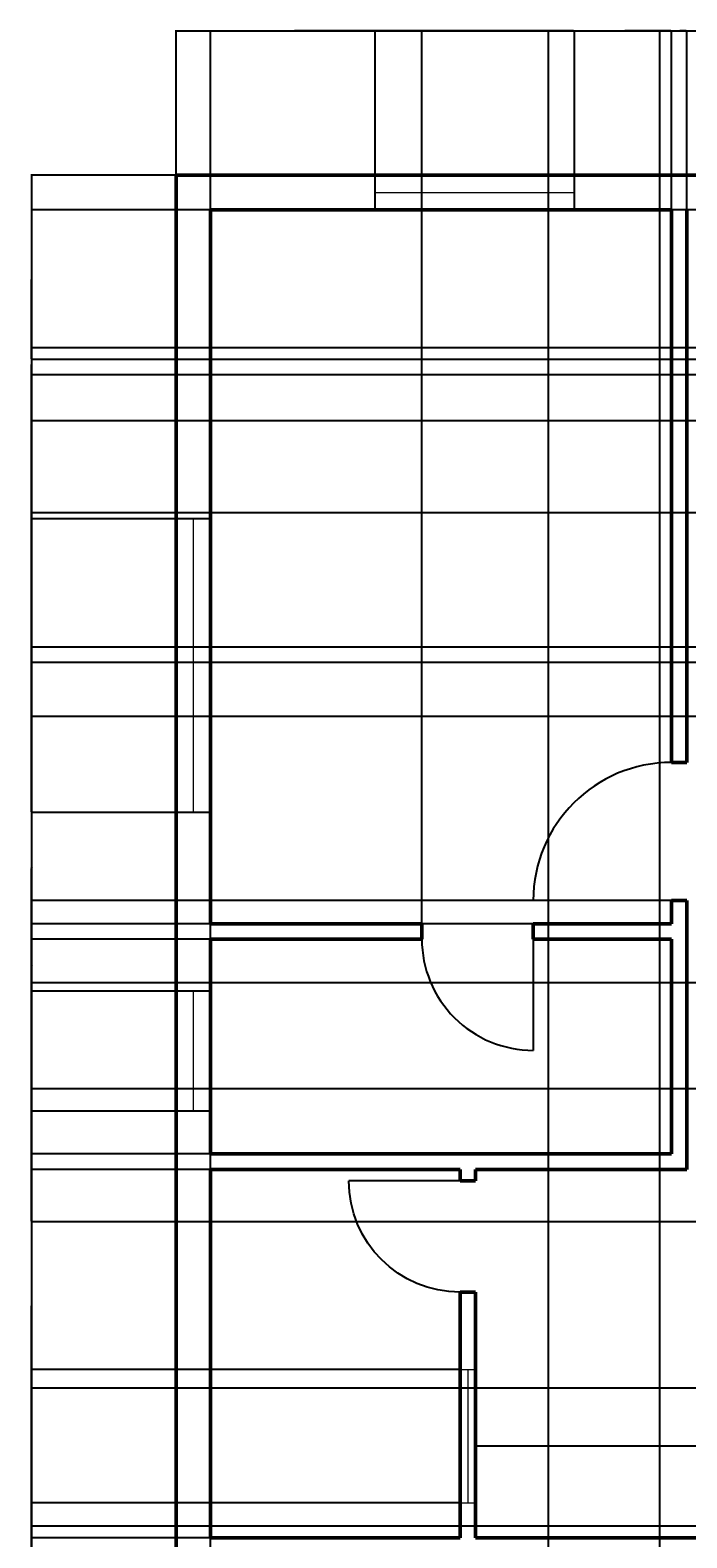
# Model space of a CAD drawing. Units: inches. Extents: x 2479 to 3284, y 2154 to 2936.
# Tile 3 of 8: x 2479 to 2650, y 2543 to 2936. Entities that reach past the tile are written whole.
import ezdxf

# ---------------------------------------------------------------- set-up
doc = ezdxf.new("R2010")
doc.units = ezdxf.units.IN
for name, color, linetype, lineweight in [('A-ANNO-DIMS', 2, 'Continuous', 18), ('A-DOOR', 3, 'Continuous', 25), ('A-FLOR-CASE', 8, 'Continuous', 18), ('A-GLAZ', 4, 'Continuous', 18), ('A-WALL', 7, 'Continuous', 50)]:
    doc.layers.add(name, color=color, linetype=linetype, lineweight=lineweight)
doc.styles.get("Standard").update_dxf_attribs({"font": 'arial.ttf'})
doc.dimstyles.get("Standard").update_dxf_attribs({"dimtxt": 0.18, "dimasz": 0.18, "dimexe": 0.18, "dimexo": 0.0625, "dimgap": 0.09, "dimtad": 0, "dimtih": 1, "dimtoh": 1, "dimdec": 4, "dimzin": 0, "dimdsep": 46, "dimtxsty": 'Standard', "dimcen": 0.09, "dimadec": 0, "dimazin": 0, "dimtfac": 1, "dimtdec": 4, "dimtofl": 0, "dimtmove": 0, "dimatfit": 3, "dimfxl": 1, "dimtolj": 1, "dimtzin": 0, "dimarcsym": 0})

# ---------------------------------------------------------------- blocks, each defined once
blk = doc.blocks.new('DOOR-SWING-29IN')
blk.add_line((29, 0), (0, 0))
blk.add_arc((29, 0), 29, 90, 180)
blk = doc.blocks.new('DOOR-SWING-36IN')
blk.add_line((36, 0), (0, 0))
blk.add_arc((36, 0), 36, 90, 180)
blk = doc.blocks.new('*D8')
at = {"layer": 'A-ANNO-DIMS', "color": 0, "lineweight": -2, "transparency": 16777216}
for p, q in [((2517.15, 2897.74), (2479.43, 2897.74)), ((2479.61, 2897.56), (2479.61, 2544.92)), ((2479.61, 2191.92), (2479.61, 2544.56)), ((2517.15, 2191.74), (2479.43, 2191.74))]:
    blk.add_line(p, q, dxfattribs=at)
at = {"layer": 'A-ANNO-DIMS', "color": 0, "transparency": 16777216}
for points in [[(2479.58, 2897.56), (2479.64, 2897.56), (2479.61, 2897.74)], [(2479.58, 2191.92), (2479.64, 2191.92), (2479.61, 2191.74)]]:
    blk.add_solid(points, dxfattribs=at)
at = {"layer": 'Defpoints', "color": 0, "transparency": 16777216}
for p in [(2479.61, 2897.74), (2517.21, 2897.74), (2517.21, 2191.74)]:
    blk.add_point(p, dxfattribs=at)
at = {"layer": 'A-ANNO-DIMS', "color": 0, "transparency": 16777216, "insert": (2479.61, 2544.74), "char_height": 0.18, "attachment_point": 5}
blk.add_mtext('\\A1;706', dxfattribs=at)
blk = doc.blocks.new('*D9')
at = {"layer": 'A-ANNO-DIMS', "color": 0, "lineweight": -2, "transparency": 16777216}
for p, q in [((2517.21, 2897.8), (2517.21, 2935.52)), ((2517.39, 2935.34), (2710.92, 2935.34)), ((2905.03, 2935.34), (2711.5, 2935.34)), ((2905.21, 2888.8), (2905.21, 2935.52))]:
    blk.add_line(p, q, dxfattribs=at)
at = {"layer": 'A-ANNO-DIMS', "color": 0, "transparency": 16777216}
for points in [[(2517.39, 2935.37), (2517.39, 2935.31), (2517.21, 2935.34)], [(2905.03, 2935.37), (2905.03, 2935.31), (2905.21, 2935.34)]]:
    blk.add_solid(points, dxfattribs=at)
at = {"layer": 'Defpoints', "color": 0, "transparency": 16777216}
for p in [(2905.21, 2935.34), (2517.21, 2897.74), (2905.21, 2888.74)]:
    blk.add_point(p, dxfattribs=at)
at = {"layer": 'A-ANNO-DIMS', "color": 0, "transparency": 16777216, "insert": (2711.21, 2935.34), "char_height": 0.18, "attachment_point": 5}
blk.add_mtext('\\A1;388', dxfattribs=at)
blk = doc.blocks.new('*D27')
at = {"layer": 'A-ANNO-DIMS', "color": 0, "lineweight": -2, "transparency": 16777216}
for p, q in [((2845.15, 2545.74), (2479.43, 2545.74)), ((2479.61, 2545.56), (2479.61, 2536.92)), ((2479.61, 2527.92), (2479.61, 2536.56)), ((2845.15, 2527.74), (2479.43, 2527.74))]:
    blk.add_line(p, q, dxfattribs=at)
at = {"layer": 'A-ANNO-DIMS', "color": 0, "transparency": 16777216}
for points in [[(2479.58, 2545.56), (2479.64, 2545.56), (2479.61, 2545.74)], [(2479.58, 2527.92), (2479.64, 2527.92), (2479.61, 2527.74)]]:
    blk.add_solid(points, dxfattribs=at)
at = {"layer": 'Defpoints', "color": 0, "transparency": 16777216}
for p in [(2479.61, 2545.74), (2845.21, 2545.74), (2845.21, 2527.74)]:
    blk.add_point(p, dxfattribs=at)
at = {"layer": 'A-ANNO-DIMS', "color": 0, "transparency": 16777216, "insert": (2479.61, 2536.74), "char_height": 0.18, "attachment_point": 5}
blk.add_mtext('\\A1;18', dxfattribs=at)
blk = doc.blocks.new('*D28')
at = {"layer": 'A-ANNO-DIMS', "color": 0, "lineweight": -2, "transparency": 16777216}
for p, q in [((2845.15, 2625.04), (2479.43, 2625.04)), ((2479.61, 2624.86), (2479.61, 2603.57)), ((2479.61, 2581.92), (2479.61, 2603.21)), ((2845.15, 2581.74), (2479.43, 2581.74))]:
    blk.add_line(p, q, dxfattribs=at)
at = {"layer": 'A-ANNO-DIMS', "color": 0, "transparency": 16777216}
for points in [[(2479.58, 2624.86), (2479.64, 2624.86), (2479.61, 2625.04)], [(2479.58, 2581.92), (2479.64, 2581.92), (2479.61, 2581.74)]]:
    blk.add_solid(points, dxfattribs=at)
at = {"layer": 'Defpoints', "color": 0, "transparency": 16777216}
for p in [(2479.61, 2625.04), (2845.21, 2625.04), (2845.21, 2581.74)]:
    blk.add_point(p, dxfattribs=at)
at = {"layer": 'A-ANNO-DIMS', "color": 0, "transparency": 16777216, "insert": (2479.61, 2603.39), "char_height": 0.18, "attachment_point": 5}
blk.add_mtext('\\A1;43.3', dxfattribs=at)
blk = doc.blocks.new('*D29')
at = {"layer": 'A-ANNO-DIMS', "color": 0, "lineweight": -2, "transparency": 16777216}
for p, q in [((2845.15, 2687.36), (2479.43, 2687.36)), ((2479.61, 2687.18), (2479.61, 2656.38)), ((2479.61, 2625.22), (2479.61, 2656.01)), ((2845.15, 2625.04), (2479.43, 2625.04))]:
    blk.add_line(p, q, dxfattribs=at)
at = {"layer": 'A-ANNO-DIMS', "color": 0, "transparency": 16777216}
for points in [[(2479.58, 2687.18), (2479.64, 2687.18), (2479.61, 2687.36)], [(2479.58, 2625.22), (2479.64, 2625.22), (2479.61, 2625.04)]]:
    blk.add_solid(points, dxfattribs=at)
at = {"layer": 'Defpoints', "color": 0, "transparency": 16777216}
for p in [(2479.61, 2687.36), (2845.21, 2687.36), (2845.21, 2625.04)]:
    blk.add_point(p, dxfattribs=at)
at = {"layer": 'A-ANNO-DIMS', "color": 0, "transparency": 16777216, "insert": (2479.61, 2656.2), "char_height": 0.18, "attachment_point": 5}
blk.add_mtext('\\A1;62.32', dxfattribs=at)
blk = doc.blocks.new('*D30')
at = {"layer": 'A-ANNO-DIMS', "color": 0, "lineweight": -2, "transparency": 16777216}
for p, q in [((2845.15, 2852.74), (2479.43, 2852.74)), ((2479.61, 2852.56), (2479.61, 2804.92)), ((2479.61, 2756.92), (2479.61, 2804.56)), ((2845.15, 2756.74), (2479.43, 2756.74))]:
    blk.add_line(p, q, dxfattribs=at)
at = {"layer": 'A-ANNO-DIMS', "color": 0, "transparency": 16777216}
for points in [[(2479.58, 2852.56), (2479.64, 2852.56), (2479.61, 2852.74)], [(2479.58, 2756.92), (2479.64, 2756.92), (2479.61, 2756.74)]]:
    blk.add_solid(points, dxfattribs=at)
at = {"layer": 'Defpoints', "color": 0, "transparency": 16777216}
for p in [(2479.61, 2852.74), (2845.21, 2852.74), (2845.21, 2756.74)]:
    blk.add_point(p, dxfattribs=at)
at = {"layer": 'A-ANNO-DIMS', "color": 0, "transparency": 16777216, "insert": (2479.61, 2804.74), "char_height": 0.18, "attachment_point": 5}
blk.add_mtext('\\A1;96', dxfattribs=at)
blk = doc.blocks.new('*D31')
at = {"layer": 'A-ANNO-DIMS', "color": 0, "lineweight": -2, "transparency": 16777216}
for p, q in [((2845.15, 2888.74), (2479.43, 2888.74)), ((2479.61, 2888.56), (2479.61, 2870.92)), ((2479.61, 2852.92), (2479.61, 2870.56)), ((2845.15, 2852.74), (2479.43, 2852.74))]:
    blk.add_line(p, q, dxfattribs=at)
at = {"layer": 'A-ANNO-DIMS', "color": 0, "transparency": 16777216}
for points in [[(2479.58, 2888.56), (2479.64, 2888.56), (2479.61, 2888.74)], [(2479.58, 2852.92), (2479.64, 2852.92), (2479.61, 2852.74)]]:
    blk.add_solid(points, dxfattribs=at)
at = {"layer": 'Defpoints', "color": 0, "transparency": 16777216}
for p in [(2479.61, 2888.74), (2845.21, 2888.74), (2845.21, 2852.74)]:
    blk.add_point(p, dxfattribs=at)
at = {"layer": 'A-ANNO-DIMS', "color": 0, "transparency": 16777216, "insert": (2479.61, 2870.74), "char_height": 0.18, "attachment_point": 5}
blk.add_mtext('\\A1;36', dxfattribs=at)
blk = doc.blocks.new('*D37')
at = {"layer": 'A-ANNO-DIMS', "color": 0, "lineweight": -2, "transparency": 16777216}
for p, q in [((2526.21, 2888.8), (2526.21, 2935.52)), ((2526.39, 2935.34), (2547.16, 2935.34)), ((2568.86, 2935.34), (2548.09, 2935.34)), ((2569.04, 2888.8), (2569.04, 2935.52))]:
    blk.add_line(p, q, dxfattribs=at)
at = {"layer": 'A-ANNO-DIMS', "color": 0, "transparency": 16777216}
for points in [[(2526.39, 2935.37), (2526.39, 2935.31), (2526.21, 2935.34)], [(2568.86, 2935.37), (2568.86, 2935.31), (2569.04, 2935.34)]]:
    blk.add_solid(points, dxfattribs=at)
at = {"layer": 'Defpoints', "color": 0, "transparency": 16777216}
for p in [(2569.04, 2935.34), (2526.21, 2888.74), (2569.04, 2888.74)]:
    blk.add_point(p, dxfattribs=at)
at = {"layer": 'A-ANNO-DIMS', "color": 0, "transparency": 16777216, "insert": (2547.63, 2935.34), "char_height": 0.18, "attachment_point": 5}
blk.add_mtext('\\A1;42.835', dxfattribs=at)
blk = doc.blocks.new('*D38')
at = {"layer": 'A-ANNO-DIMS', "color": 0, "lineweight": -2, "transparency": 16777216}
for p, q in [((2569.04, 2888.8), (2569.04, 2935.52)), ((2569.22, 2935.34), (2594.59, 2935.34)), ((2620.74, 2935.34), (2595.38, 2935.34)), ((2620.92, 2888.8), (2620.92, 2935.52))]:
    blk.add_line(p, q, dxfattribs=at)
at = {"layer": 'A-ANNO-DIMS', "color": 0, "transparency": 16777216}
for points in [[(2569.22, 2935.37), (2569.22, 2935.31), (2569.04, 2935.34)], [(2620.74, 2935.37), (2620.74, 2935.31), (2620.92, 2935.34)]]:
    blk.add_solid(points, dxfattribs=at)
at = {"layer": 'Defpoints', "color": 0, "transparency": 16777216}
for p in [(2620.92, 2935.34), (2569.04, 2888.74), (2620.92, 2888.74)]:
    blk.add_point(p, dxfattribs=at)
at = {"layer": 'A-ANNO-DIMS', "color": 0, "transparency": 16777216, "insert": (2594.98, 2935.34), "char_height": 0.18, "attachment_point": 5}
blk.add_mtext('\\A1;51.88', dxfattribs=at)
blk = doc.blocks.new('*D39')
at = {"layer": 'A-ANNO-DIMS', "color": 0, "lineweight": -2, "transparency": 16777216}
for p, q in [((2620.92, 2888.8), (2620.92, 2935.52)), ((2621.1, 2935.34), (2633.1, 2935.34)), ((2646.03, 2935.34), (2634.03, 2935.34)), ((2646.21, 2888.8), (2646.21, 2935.52))]:
    blk.add_line(p, q, dxfattribs=at)
at = {"layer": 'A-ANNO-DIMS', "color": 0, "transparency": 16777216}
for points in [[(2621.1, 2935.37), (2621.1, 2935.31), (2620.92, 2935.34)], [(2646.03, 2935.37), (2646.03, 2935.31), (2646.21, 2935.34)]]:
    blk.add_solid(points, dxfattribs=at)
at = {"layer": 'Defpoints', "color": 0, "transparency": 16777216}
for p in [(2646.21, 2935.34), (2620.92, 2888.74), (2646.21, 2888.74)]:
    blk.add_point(p, dxfattribs=at)
at = {"layer": 'A-ANNO-DIMS', "color": 0, "transparency": 16777216, "insert": (2633.57, 2935.34), "char_height": 0.18, "attachment_point": 5}
blk.add_mtext('\\A1;25.285', dxfattribs=at)
blk = doc.blocks.new('*D40')
at = {"layer": 'A-ANNO-DIMS', "color": 0, "lineweight": -2, "transparency": 16777216}
for p, q in [((2646.21, 2888.8), (2646.21, 2935.52)), ((2646.39, 2935.34), (2648.06, 2935.34)), ((2650.03, 2935.34), (2648.36, 2935.34)), ((2650.21, 2888.8), (2650.21, 2935.52))]:
    blk.add_line(p, q, dxfattribs=at)
at = {"layer": 'A-ANNO-DIMS', "color": 0, "transparency": 16777216}
for points in [[(2646.39, 2935.37), (2646.39, 2935.31), (2646.21, 2935.34)], [(2650.03, 2935.37), (2650.03, 2935.31), (2650.21, 2935.34)]]:
    blk.add_solid(points, dxfattribs=at)
at = {"layer": 'Defpoints', "color": 0, "transparency": 16777216}
for p in [(2650.21, 2935.34), (2646.21, 2888.74), (2650.21, 2888.74)]:
    blk.add_point(p, dxfattribs=at)
at = {"layer": 'A-ANNO-DIMS', "color": 0, "transparency": 16777216, "insert": (2648.21, 2935.34), "char_height": 0.18, "attachment_point": 5}
blk.add_mtext('\\A1;4', dxfattribs=at)
blk = doc.blocks.new('*D51')
at = {"layer": 'A-ANNO-DIMS', "color": 0, "lineweight": -2, "transparency": 16777216}
for p, q in [((2526.15, 2638.74), (2479.43, 2638.74)), ((2479.61, 2638.56), (2479.61, 2590.92)), ((2479.61, 2542.92), (2479.61, 2590.56)), ((2526.15, 2542.74), (2479.43, 2542.74))]:
    blk.add_line(p, q, dxfattribs=at)
at = {"layer": 'A-ANNO-DIMS', "color": 0, "transparency": 16777216}
for points in [[(2479.58, 2638.56), (2479.64, 2638.56), (2479.61, 2638.74)], [(2479.58, 2542.92), (2479.64, 2542.92), (2479.61, 2542.74)]]:
    blk.add_solid(points, dxfattribs=at)
at = {"layer": 'Defpoints', "color": 0, "transparency": 16777216}
for p in [(2479.61, 2638.74), (2526.21, 2638.74), (2526.21, 2542.74)]:
    blk.add_point(p, dxfattribs=at)
at = {"layer": 'A-ANNO-DIMS', "color": 0, "transparency": 16777216, "insert": (2479.61, 2590.74), "char_height": 0.18, "attachment_point": 5}
blk.add_mtext('\\A1;96', dxfattribs=at)
blk = doc.blocks.new('*D52')
at = {"layer": 'A-ANNO-DIMS', "color": 0, "lineweight": -2, "transparency": 16777216}
for p, q in [((2526.15, 2653.92), (2479.43, 2653.92)), ((2479.61, 2653.74), (2479.61, 2648.51)), ((2479.61, 2642.92), (2479.61, 2648.15)), ((2526.15, 2642.74), (2479.43, 2642.74))]:
    blk.add_line(p, q, dxfattribs=at)
at = {"layer": 'A-ANNO-DIMS', "color": 0, "transparency": 16777216}
for points in [[(2479.58, 2653.74), (2479.64, 2653.74), (2479.61, 2653.92)], [(2479.58, 2642.92), (2479.64, 2642.92), (2479.61, 2642.74)]]:
    blk.add_solid(points, dxfattribs=at)
at = {"layer": 'Defpoints', "color": 0, "transparency": 16777216}
for p in [(2479.61, 2653.92), (2526.21, 2653.92), (2526.21, 2642.74)]:
    blk.add_point(p, dxfattribs=at)
at = {"layer": 'A-ANNO-DIMS', "color": 0, "transparency": 16777216, "insert": (2479.61, 2648.33), "char_height": 0.18, "attachment_point": 5}
blk.add_mtext('\\A1;11.18', dxfattribs=at)
blk = doc.blocks.new('*D53')
at = {"layer": 'A-ANNO-DIMS', "color": 0, "lineweight": -2, "transparency": 16777216}
for p, q in [((2526.15, 2685.18), (2479.43, 2685.18)), ((2479.61, 2685), (2479.61, 2669.73)), ((2479.61, 2654.1), (2479.61, 2669.37)), ((2526.15, 2653.92), (2479.43, 2653.92))]:
    blk.add_line(p, q, dxfattribs=at)
at = {"layer": 'A-ANNO-DIMS', "color": 0, "transparency": 16777216}
for points in [[(2479.58, 2685), (2479.64, 2685), (2479.61, 2685.18)], [(2479.58, 2654.1), (2479.64, 2654.1), (2479.61, 2653.92)]]:
    blk.add_solid(points, dxfattribs=at)
at = {"layer": 'Defpoints', "color": 0, "transparency": 16777216}
for p in [(2479.61, 2685.18), (2526.21, 2685.18), (2526.21, 2653.92)]:
    blk.add_point(p, dxfattribs=at)
at = {"layer": 'A-ANNO-DIMS', "color": 0, "transparency": 16777216, "insert": (2479.61, 2669.55), "char_height": 0.18, "attachment_point": 5}
blk.add_mtext('\\A1;31.26', dxfattribs=at)
blk = doc.blocks.new('*D54')
at = {"layer": 'A-ANNO-DIMS', "color": 0, "lineweight": -2, "transparency": 16777216}
for p, q in [((2526.15, 2698.74), (2479.43, 2698.74)), ((2479.61, 2698.56), (2479.61, 2692.14)), ((2479.61, 2685.36), (2479.61, 2691.78)), ((2526.15, 2685.18), (2479.43, 2685.18))]:
    blk.add_line(p, q, dxfattribs=at)
at = {"layer": 'A-ANNO-DIMS', "color": 0, "transparency": 16777216}
for points in [[(2479.58, 2698.56), (2479.64, 2698.56), (2479.61, 2698.74)], [(2479.58, 2685.36), (2479.64, 2685.36), (2479.61, 2685.18)]]:
    blk.add_solid(points, dxfattribs=at)
at = {"layer": 'Defpoints', "color": 0, "transparency": 16777216}
for p in [(2479.61, 2698.74), (2526.21, 2698.74), (2526.21, 2685.18)]:
    blk.add_point(p, dxfattribs=at)
at = {"layer": 'A-ANNO-DIMS', "color": 0, "transparency": 16777216, "insert": (2479.61, 2691.96), "char_height": 0.18, "attachment_point": 5}
blk.add_mtext('\\A1;13.557', dxfattribs=at)
blk = doc.blocks.new('*D55')
at = {"layer": 'A-ANNO-DIMS', "color": 0, "lineweight": -2, "transparency": 16777216}
for p, q in [((2526.15, 2731.68), (2479.43, 2731.68)), ((2479.61, 2731.5), (2479.61, 2717.39)), ((2479.61, 2702.92), (2479.61, 2717.03)), ((2526.15, 2702.74), (2479.43, 2702.74))]:
    blk.add_line(p, q, dxfattribs=at)
at = {"layer": 'A-ANNO-DIMS', "color": 0, "transparency": 16777216}
for points in [[(2479.58, 2731.5), (2479.64, 2731.5), (2479.61, 2731.68)], [(2479.58, 2702.92), (2479.64, 2702.92), (2479.61, 2702.74)]]:
    blk.add_solid(points, dxfattribs=at)
at = {"layer": 'Defpoints', "color": 0, "transparency": 16777216}
for p in [(2479.61, 2731.68), (2526.21, 2731.68), (2526.21, 2702.74)]:
    blk.add_point(p, dxfattribs=at)
at = {"layer": 'A-ANNO-DIMS', "color": 0, "transparency": 16777216, "insert": (2479.61, 2717.21), "char_height": 0.18, "attachment_point": 5}
blk.add_mtext('\\A1;28.935', dxfattribs=at)
blk = doc.blocks.new('*D56')
at = {"layer": 'A-ANNO-DIMS', "color": 0, "lineweight": -2, "transparency": 16777216}
for p, q in [((2526.15, 2808.2), (2479.43, 2808.2)), ((2479.61, 2808.02), (2479.61, 2770.12)), ((2479.61, 2731.86), (2479.61, 2769.75)), ((2526.15, 2731.68), (2479.43, 2731.68))]:
    blk.add_line(p, q, dxfattribs=at)
at = {"layer": 'A-ANNO-DIMS', "color": 0, "transparency": 16777216}
for points in [[(2479.58, 2808.02), (2479.64, 2808.02), (2479.61, 2808.2)], [(2479.58, 2731.86), (2479.64, 2731.86), (2479.61, 2731.68)]]:
    blk.add_solid(points, dxfattribs=at)
at = {"layer": 'Defpoints', "color": 0, "transparency": 16777216}
for p in [(2479.61, 2808.2), (2526.21, 2808.2), (2526.21, 2731.68)]:
    blk.add_point(p, dxfattribs=at)
at = {"layer": 'A-ANNO-DIMS', "color": 0, "transparency": 16777216, "insert": (2479.61, 2769.94), "char_height": 0.18, "attachment_point": 5}
blk.add_mtext('\\A1;76.52', dxfattribs=at)
blk = doc.blocks.new('*D57')
at = {"layer": 'A-ANNO-DIMS', "color": 0, "lineweight": -2, "transparency": 16777216}
for p, q in [((2526.15, 2888.74), (2479.43, 2888.74)), ((2479.61, 2888.56), (2479.61, 2848.65)), ((2479.61, 2808.38), (2479.61, 2848.29)), ((2526.15, 2808.2), (2479.43, 2808.2))]:
    blk.add_line(p, q, dxfattribs=at)
at = {"layer": 'A-ANNO-DIMS', "color": 0, "transparency": 16777216}
for points in [[(2479.58, 2888.56), (2479.64, 2888.56), (2479.61, 2888.74)], [(2479.58, 2808.38), (2479.64, 2808.38), (2479.61, 2808.2)]]:
    blk.add_solid(points, dxfattribs=at)
at = {"layer": 'Defpoints', "color": 0, "transparency": 16777216}
for p in [(2479.61, 2888.74), (2526.21, 2888.74), (2526.21, 2808.2)]:
    blk.add_point(p, dxfattribs=at)
at = {"layer": 'A-ANNO-DIMS', "color": 0, "transparency": 16777216, "insert": (2479.61, 2848.47), "char_height": 0.18, "attachment_point": 5}
blk.add_mtext('\\A1;80.54', dxfattribs=at)
blk = doc.blocks.new('*D61')
at = {"layer": 'A-ANNO-DIMS', "color": 0, "lineweight": -2, "transparency": 16777216}
for p, q in [((2595.27, 2566.74), (3283.99, 2566.74)), ((3283.81, 2566.56), (3283.81, 2554.92)), ((3283.81, 2542.92), (3283.81, 2554.56)), ((2595.27, 2542.74), (3283.99, 2542.74))]:
    blk.add_line(p, q, dxfattribs=at)
at = {"layer": 'A-ANNO-DIMS', "color": 0, "transparency": 16777216}
for points in [[(3283.78, 2566.56), (3283.84, 2566.56), (3283.81, 2566.74)], [(3283.78, 2542.92), (3283.84, 2542.92), (3283.81, 2542.74)]]:
    blk.add_solid(points, dxfattribs=at)
at = {"layer": 'Defpoints', "color": 0, "transparency": 16777216}
for p in [(2595.21, 2566.74), (3283.81, 2566.74), (2595.21, 2542.74)]:
    blk.add_point(p, dxfattribs=at)
at = {"layer": 'A-ANNO-DIMS', "color": 0, "transparency": 16777216, "insert": (3283.81, 2554.74), "char_height": 0.18, "attachment_point": 5}
blk.add_mtext('\\A1;24', dxfattribs=at)
blk = doc.blocks.new('*D62')
at = {"layer": 'A-ANNO-DIMS', "color": 0, "lineweight": -2, "transparency": 16777216}
for p, q in [((2591.15, 2586.56), (2479.43, 2586.56)), ((2479.61, 2586.38), (2479.61, 2569.41)), ((2479.61, 2552.08), (2479.61, 2569.05)), ((2591.15, 2551.9), (2479.43, 2551.9))]:
    blk.add_line(p, q, dxfattribs=at)
at = {"layer": 'A-ANNO-DIMS', "color": 0, "transparency": 16777216}
for points in [[(2479.58, 2586.38), (2479.64, 2586.38), (2479.61, 2586.56)], [(2479.58, 2552.08), (2479.64, 2552.08), (2479.61, 2551.9)]]:
    blk.add_solid(points, dxfattribs=at)
at = {"layer": 'Defpoints', "color": 0, "transparency": 16777216}
for p in [(2479.61, 2586.56), (2591.21, 2586.56), (2591.21, 2551.9)]:
    blk.add_point(p, dxfattribs=at)
at = {"layer": 'A-ANNO-DIMS', "color": 0, "transparency": 16777216, "insert": (2479.61, 2569.23), "char_height": 0.18, "attachment_point": 5}
blk.add_mtext('\\A1;34.66', dxfattribs=at)
blk = doc.blocks.new('*D64')
at = {"layer": 'A-ANNO-DIMS', "color": 0, "lineweight": -2, "transparency": 16777216}
for p, q in [((2526.21, 2698.8), (2526.21, 2935.52)), ((2526.39, 2935.34), (2553.49, 2935.34)), ((2581.03, 2935.34), (2553.93, 2935.34)), ((2581.21, 2698.8), (2581.21, 2935.52))]:
    blk.add_line(p, q, dxfattribs=at)
at = {"layer": 'A-ANNO-DIMS', "color": 0, "transparency": 16777216}
for points in [[(2526.39, 2935.37), (2526.39, 2935.31), (2526.21, 2935.34)], [(2581.03, 2935.37), (2581.03, 2935.31), (2581.21, 2935.34)]]:
    blk.add_solid(points, dxfattribs=at)
at = {"layer": 'Defpoints', "color": 0, "transparency": 16777216}
for p in [(2581.21, 2935.34), (2526.21, 2698.74), (2581.21, 2698.74)]:
    blk.add_point(p, dxfattribs=at)
at = {"layer": 'A-ANNO-DIMS', "color": 0, "transparency": 16777216, "insert": (2553.71, 2935.34), "char_height": 0.18, "attachment_point": 5}
blk.add_mtext('\\A1;55', dxfattribs=at)
blk = doc.blocks.new('*D65')
at = {"layer": 'A-ANNO-DIMS', "color": 0, "lineweight": -2, "transparency": 16777216}
for p, q in [((2646.15, 2708.74), (2479.43, 2708.74)), ((2479.61, 2708.56), (2479.61, 2705.92)), ((2646.15, 2702.74), (2479.43, 2702.74)), ((2479.61, 2702.92), (2479.61, 2705.56))]:
    blk.add_line(p, q, dxfattribs=at)
at = {"layer": 'A-ANNO-DIMS', "color": 0, "transparency": 16777216}
for points in [[(2479.58, 2708.56), (2479.64, 2708.56), (2479.61, 2708.74)], [(2479.58, 2702.92), (2479.64, 2702.92), (2479.61, 2702.74)]]:
    blk.add_solid(points, dxfattribs=at)
at = {"layer": 'Defpoints', "color": 0, "transparency": 16777216}
for p in [(2479.61, 2708.74), (2646.21, 2708.74), (2646.21, 2702.74)]:
    blk.add_point(p, dxfattribs=at)
at = {"layer": 'A-ANNO-DIMS', "color": 0, "transparency": 16777216, "insert": (2479.61, 2705.74), "char_height": 0.18, "attachment_point": 5}
blk.add_mtext('\\A1;6', dxfattribs=at)
blk = doc.blocks.new('*D84')
at = {"layer": 'A-ANNO-DIMS', "color": 0, "lineweight": -2, "transparency": 16777216}
for p, q in [((3032.15, 2888.74), (2479.43, 2888.74)), ((2479.61, 2888.56), (2479.61, 2869.42)), ((2479.61, 2849.92), (2479.61, 2869.06)), ((3032.15, 2849.74), (2479.43, 2849.74))]:
    blk.add_line(p, q, dxfattribs=at)
at = {"layer": 'A-ANNO-DIMS', "color": 0, "transparency": 16777216}
for points in [[(2479.58, 2888.56), (2479.64, 2888.56), (2479.61, 2888.74)], [(2479.58, 2849.92), (2479.64, 2849.92), (2479.61, 2849.74)]]:
    blk.add_solid(points, dxfattribs=at)
at = {"layer": 'Defpoints', "color": 0, "transparency": 16777216}
for p in [(2479.61, 2888.74), (3032.21, 2888.74), (3032.21, 2849.74)]:
    blk.add_point(p, dxfattribs=at)
at = {"layer": 'A-ANNO-DIMS', "color": 0, "transparency": 16777216, "insert": (2479.61, 2869.24), "char_height": 0.18, "attachment_point": 5}
blk.add_mtext('\\A1;39', dxfattribs=at)
blk = doc.blocks.new('*D85')
at = {"layer": 'A-ANNO-DIMS', "color": 0, "lineweight": -2, "transparency": 16777216}
for p, q in [((2911.15, 2845.74), (2479.43, 2845.74)), ((2479.61, 2845.56), (2479.61, 2810.42)), ((2479.61, 2774.92), (2479.61, 2810.06)), ((3041.15, 2774.74), (2479.43, 2774.74))]:
    blk.add_line(p, q, dxfattribs=at)
at = {"layer": 'A-ANNO-DIMS', "color": 0, "transparency": 16777216}
for points in [[(2479.58, 2845.56), (2479.64, 2845.56), (2479.61, 2845.74)], [(2479.58, 2774.92), (2479.64, 2774.92), (2479.61, 2774.74)]]:
    blk.add_solid(points, dxfattribs=at)
at = {"layer": 'Defpoints', "color": 0, "transparency": 16777216}
for p in [(2479.61, 2845.74), (2911.21, 2845.74), (3041.21, 2774.74)]:
    blk.add_point(p, dxfattribs=at)
at = {"layer": 'A-ANNO-DIMS', "color": 0, "transparency": 16777216, "insert": (2479.61, 2810.24), "char_height": 0.18, "attachment_point": 5}
blk.add_mtext('\\A1;71', dxfattribs=at)
blk = doc.blocks.new('*D86')
at = {"layer": 'A-ANNO-DIMS', "color": 0, "lineweight": -2, "transparency": 16777216}
for p, q in [((3041.15, 2770.74), (2479.43, 2770.74)), ((2479.61, 2770.56), (2479.61, 2715.42)), ((2479.61, 2659.92), (2479.61, 2715.06)), ((2911.15, 2659.74), (2479.43, 2659.74))]:
    blk.add_line(p, q, dxfattribs=at)
at = {"layer": 'A-ANNO-DIMS', "color": 0, "transparency": 16777216}
for points in [[(2479.58, 2770.56), (2479.64, 2770.56), (2479.61, 2770.74)], [(2479.58, 2659.92), (2479.64, 2659.92), (2479.61, 2659.74)]]:
    blk.add_solid(points, dxfattribs=at)
at = {"layer": 'Defpoints', "color": 0, "transparency": 16777216}
for p in [(2479.61, 2770.74), (3041.21, 2770.74), (2911.21, 2659.74)]:
    blk.add_point(p, dxfattribs=at)
at = {"layer": 'A-ANNO-DIMS', "color": 0, "transparency": 16777216, "insert": (2479.61, 2715.24), "char_height": 0.18, "attachment_point": 5}
blk.add_mtext('\\A1;111', dxfattribs=at)
blk = doc.blocks.new('*D89')
at = {"layer": 'A-ANNO-DIMS', "color": 0, "lineweight": -2, "transparency": 16777216}
for p, q in [((3139.15, 2833.74), (2479.43, 2833.74)), ((2479.61, 2833.56), (2479.61, 2821.92)), ((2479.61, 2809.92), (2479.61, 2821.56)), ((3213.15, 2809.74), (2479.43, 2809.74))]:
    blk.add_line(p, q, dxfattribs=at)
at = {"layer": 'A-ANNO-DIMS', "color": 0, "transparency": 16777216}
for points in [[(2479.58, 2833.56), (2479.64, 2833.56), (2479.61, 2833.74)], [(2479.58, 2809.92), (2479.64, 2809.92), (2479.61, 2809.74)]]:
    blk.add_solid(points, dxfattribs=at)
at = {"layer": 'Defpoints', "color": 0, "transparency": 16777216}
for p in [(2479.61, 2833.74), (3139.21, 2833.74), (3213.21, 2809.74)]:
    blk.add_point(p, dxfattribs=at)
at = {"layer": 'A-ANNO-DIMS', "color": 0, "transparency": 16777216, "insert": (2479.61, 2821.74), "char_height": 0.18, "attachment_point": 5}
blk.add_mtext('\\A1;24', dxfattribs=at)
blk = doc.blocks.new('*D109')
at = {"layer": 'A-ANNO-DIMS', "color": 0, "lineweight": -2, "transparency": 16777216}
for p, q in [((2526.21, 2407.8), (2526.21, 2935.52)), ((2526.39, 2935.34), (2569.99, 2935.34)), ((2614.03, 2935.34), (2570.43, 2935.34)), ((2614.21, 2407.8), (2614.21, 2935.52))]:
    blk.add_line(p, q, dxfattribs=at)
at = {"layer": 'A-ANNO-DIMS', "color": 0, "transparency": 16777216}
for points in [[(2526.39, 2935.37), (2526.39, 2935.31), (2526.21, 2935.34)], [(2614.03, 2935.37), (2614.03, 2935.31), (2614.21, 2935.34)]]:
    blk.add_solid(points, dxfattribs=at)
at = {"layer": 'Defpoints', "color": 0, "transparency": 16777216}
for p in [(2614.21, 2935.34), (2526.21, 2407.74), (2614.21, 2407.74)]:
    blk.add_point(p, dxfattribs=at)
at = {"layer": 'A-ANNO-DIMS', "color": 0, "transparency": 16777216, "insert": (2570.21, 2935.34), "char_height": 0.18, "attachment_point": 5}
blk.add_mtext('\\A1;88', dxfattribs=at)
blk = doc.blocks.new('*D110')
at = {"layer": 'A-ANNO-DIMS', "color": 0, "lineweight": -2, "transparency": 16777216}
for p, q in [((2643.21, 2407.8), (2643.21, 2935.52)), ((2643.39, 2935.34), (2662.49, 2935.34)), ((2682.03, 2935.34), (2662.93, 2935.34)), ((2682.21, 2407.8), (2682.21, 2935.52))]:
    blk.add_line(p, q, dxfattribs=at)
at = {"layer": 'A-ANNO-DIMS', "color": 0, "transparency": 16777216}
for points in [[(2643.39, 2935.37), (2643.39, 2935.31), (2643.21, 2935.34)], [(2682.03, 2935.37), (2682.03, 2935.31), (2682.21, 2935.34)]]:
    blk.add_solid(points, dxfattribs=at)
at = {"layer": 'Defpoints', "color": 0, "transparency": 16777216}
for p in [(2682.21, 2935.34), (2643.21, 2407.74), (2682.21, 2407.74)]:
    blk.add_point(p, dxfattribs=at)
at = {"layer": 'A-ANNO-DIMS', "color": 0, "transparency": 16777216, "insert": (2662.71, 2935.34), "char_height": 0.18, "attachment_point": 5}
blk.add_mtext('\\A1;39', dxfattribs=at)

msp = doc.modelspace()

# ---------------------------------------------------------------- linework, layer by layer
at = {"layer": 'A-FLOR-CASE'}
msp.add_line((2697.2088, 2566.7397), (2595.2088, 2566.7397), dxfattribs=at)
at = {"layer": 'A-GLAZ'}
for p, q in [((2569.0438, 2888.7397), (2569.0438, 2897.7397)), ((2620.9238, 2888.7397), (2620.9238, 2897.7397)), ((2569.0438, 2893.2397), (2620.9238, 2893.2397)), ((2526.2088, 2808.1977), (2517.2088, 2808.1977)), ((2521.7088, 2808.1977), (2521.7088, 2731.6752)), ((2526.2088, 2731.6752), (2517.2088, 2731.6752)), ((2526.2088, 2685.1829), (2517.2088, 2685.1829)), ((2521.7088, 2685.1829), (2521.7088, 2653.9198)), ((2526.2088, 2653.9198), (2517.2088, 2653.9198)), ((2591.2088, 2586.5584), (2595.2088, 2586.5584)), ((2593.2088, 2586.5584), (2593.2088, 2551.8964)), ((2591.2088, 2551.8964), (2595.2088, 2551.8964))]:
    msp.add_line(p, q, dxfattribs=at)
at = {"layer": 'A-WALL'}
for p, q in [((3246.2088, 2897.7397), (2517.2088, 2897.7397)), ((2517.2088, 2897.7397), (2517.2088, 2191.7397)), ((2526.2088, 2888.7397), (2526.2088, 2702.7397)), ((2646.2088, 2888.7397), (2526.2088, 2888.7397)), ((2646.2088, 2888.7397), (2646.2088, 2744.7397)), ((2650.2088, 2888.7397), (2650.2088, 2744.7397)), ((2646.2088, 2744.7397), (2650.2088, 2744.7397)), ((2646.2088, 2708.7397), (2650.2088, 2708.7397)), ((2646.2088, 2708.7397), (2646.2088, 2702.7397)), ((2650.2088, 2708.7397), (2650.2088, 2642.7397)), ((2581.2088, 2702.7397), (2526.2088, 2702.7397)), ((2581.2088, 2702.7397), (2581.2088, 2698.7397)), ((2646.2088, 2702.7397), (2610.2088, 2702.7397)), ((2610.2088, 2702.7397), (2610.2088, 2698.7397)), ((2526.2088, 2698.7397), (2526.2088, 2642.7397)), ((2581.2088, 2698.7397), (2526.2088, 2698.7397)), ((2646.2088, 2698.7397), (2610.2088, 2698.7397)), ((2646.2088, 2698.7397), (2646.2088, 2642.7397)), ((2646.2088, 2642.7397), (2526.2088, 2642.7397)), ((2650.2088, 2642.7397), (2650.2088, 2638.7397)), ((2526.2088, 2638.7397), (2526.2088, 2542.7397)), ((2591.2088, 2638.7397), (2526.2088, 2638.7397)), ((2591.2088, 2638.7397), (2591.2088, 2635.7397)), ((2591.2088, 2635.7397), (2595.2088, 2635.7397)), ((2595.2088, 2638.7397), (2595.2088, 2635.7397)), ((2650.2088, 2638.7397), (2595.2088, 2638.7397)), ((2591.2088, 2606.7397), (2595.2088, 2606.7397)), ((2591.2088, 2606.7397), (2591.2088, 2542.7397)), ((2595.2088, 2606.7397), (2595.2088, 2542.7397)), ((2591.2088, 2542.7397), (2526.2088, 2542.7397)), ((2721.2088, 2542.7397), (2595.2088, 2542.7397))]:
    msp.add_line(p, q, dxfattribs=at)

# ---------------------------------------------------------------- block references
at = {"layer": 'A-DOOR'}
msp.add_blockref('DOOR-SWING-36IN', (2610.2088, 2708.7397), dxfattribs=at)
at = {"layer": 'A-DOOR', "rotation": 90.0000000000027}
msp.add_blockref('DOOR-SWING-29IN', (2610.2088, 2669.7397), dxfattribs=at)
at = {"layer": 'A-DOOR', "extrusion": (0, 0, -1), "zscale": -1, "rotation": 180}
msp.add_blockref('DOOR-SWING-29IN', (-2562.2088, 2635.7397), dxfattribs=at)

# ---------------------------------------------------------------- dimensions: what is measured, and where the dimension line sits
at = {"layer": 'A-ANNO-DIMS'}
for base, p1, p2, override, picture, middle in [((2905.2088, 2935.3397), (2517.2088, 2897.7397), (2905.2088, 2888.7397), {"dimdec": 0, "dimlfac": 1, "dimrnd": 0, "dimzin": 0, "dimdsep": 46, "dimlunit": 2}, '*D9', (2711.2088, 2935.3397)), ((2569.0438, 2935.3397), (2526.2088, 2888.7397), (2569.0438, 2888.7397), {"dimdec": 3, "dimlfac": 1, "dimrnd": 0, "dimzin": 0, "dimdsep": 46, "dimlunit": 2}, '*D37', (2547.6263, 2935.3397)), ((2581.2088, 2935.3397), (2526.2088, 2698.7397), (2581.2088, 2698.7397), {"dimdec": 0, "dimlfac": 1, "dimrnd": 0, "dimzin": 0, "dimdsep": 46, "dimlunit": 2}, '*D64', (2553.7088, 2935.3397)), ((2614.2088, 2935.3397), (2526.2088, 2407.7397), (2614.2088, 2407.7397), {"dimdec": 0, "dimlfac": 1, "dimrnd": 0, "dimzin": 0, "dimdsep": 46, "dimlunit": 2}, '*D109', (2570.2088, 2935.3397)), ((2620.9238, 2935.3397), (2569.0438, 2888.7397), (2620.9238, 2888.7397), {"dimdec": 2, "dimlfac": 1, "dimrnd": 0, "dimzin": 0, "dimdsep": 46, "dimlunit": 2}, '*D38', (2594.9838, 2935.3397)), ((2646.2088, 2935.3397), (2620.9238, 2888.7397), (2646.2088, 2888.7397), {"dimdec": 3, "dimlfac": 1, "dimrnd": 0, "dimzin": 0, "dimdsep": 46, "dimlunit": 2}, '*D39', (2633.5663, 2935.3397)), ((2682.2088, 2935.3397), (2643.2088, 2407.7397), (2682.2088, 2407.7397), {"dimdec": 0, "dimlfac": 1, "dimrnd": 0, "dimzin": 0, "dimdsep": 46, "dimlunit": 2}, '*D110', (2662.7088, 2935.3397)), ((2650.2088, 2935.3397), (2646.2088, 2888.7397), (2650.2088, 2888.7397), {"dimdec": 0, "dimlfac": 1, "dimrnd": 0, "dimzin": 0, "dimdsep": 46, "dimlunit": 2}, '*D40', (2648.2088, 2935.3397))]:
    dim = msp.add_linear_dim(base=base, p1=p1, p2=p2, dimstyle='Standard', override=override, dxfattribs=at)
    dim.commit()
    dim.dimension.update_dxf_attribs({"geometry": picture, "text_midpoint": middle})
for base, p1, p2, override, picture, middle in [((2479.6088, 2897.7397), (2517.2088, 2191.7397), (2517.2088, 2897.7397), {"dimdec": 0, "dimlfac": 1, "dimrnd": 0, "dimzin": 0, "dimdsep": 46, "dimlunit": 2}, '*D8', (2479.6088, 2544.7397)), ((2479.6088, 2888.7397), (2526.2088, 2808.1977), (2526.2088, 2888.7397), {"dimdec": 2, "dimlfac": 1, "dimrnd": 0, "dimzin": 0, "dimdsep": 46, "dimlunit": 2}, '*D57', (2479.6088, 2848.4687)), ((2479.6088, 2888.7397), (2845.2088, 2852.7397), (2845.2088, 2888.7397), {"dimdec": 0, "dimlfac": 1, "dimrnd": 0, "dimzin": 0, "dimdsep": 46, "dimlunit": 2}, '*D31', (2479.6088, 2870.7397)), ((2479.6088, 2888.7397), (3032.2088, 2849.7397), (3032.2088, 2888.7397), {"dimdec": 0, "dimlfac": 1, "dimrnd": 0, "dimzin": 0, "dimdsep": 46, "dimlunit": 2}, '*D84', (2479.6088, 2869.2397)), ((2479.6088, 2852.7397), (2845.2088, 2756.7397), (2845.2088, 2852.7397), {"dimdec": 0, "dimlfac": 1, "dimrnd": 0, "dimzin": 0, "dimdsep": 46, "dimlunit": 2}, '*D30', (2479.6088, 2804.7397)), ((2479.6088, 2845.7397), (3041.2088, 2774.7397), (2911.2088, 2845.7397), {"dimdec": 0, "dimlfac": 1, "dimrnd": 0, "dimzin": 0, "dimdsep": 46, "dimlunit": 2}, '*D85', (2479.6088, 2810.2397)), ((2479.6088, 2833.7397), (3213.2088, 2809.7397), (3139.2088, 2833.7397), {"dimdec": 0, "dimlfac": 1, "dimrnd": 0, "dimzin": 0, "dimdsep": 46, "dimlunit": 2}, '*D89', (2479.6088, 2821.7397)), ((2479.6088, 2808.1977), (2526.2088, 2731.6752), (2526.2088, 2808.1977), {"dimdec": 2, "dimlfac": 1, "dimrnd": 0, "dimzin": 0, "dimdsep": 46, "dimlunit": 2}, '*D56', (2479.6088, 2769.9365)), ((2479.6088, 2770.7397), (2911.2088, 2659.7397), (3041.2088, 2770.7397), {"dimdec": 0, "dimlfac": 1, "dimrnd": 0, "dimzin": 0, "dimdsep": 46, "dimlunit": 2}, '*D86', (2479.6088, 2715.2397)), ((2479.60882, 2731.675247), (2526.20882, 2702.739749), (2526.20882, 2731.675247), {"dimdec": 3, "dimlfac": 1, "dimrnd": 0, "dimzin": 0, "dimdsep": 46, "dimlunit": 2}, '*D55', (2479.60882, 2717.207498)), ((2479.6088, 2708.7397), (2646.2088, 2702.7397), (2646.2088, 2708.7397), {"dimdec": 0, "dimlfac": 1, "dimrnd": 0, "dimzin": 0, "dimdsep": 46, "dimlunit": 2}, '*D65', (2479.6088, 2705.7397)), ((2479.6088, 2698.7397), (2526.2088, 2685.1829), (2526.2088, 2698.7397), {"dimdec": 3, "dimlfac": 1, "dimrnd": 0, "dimzin": 0, "dimdsep": 46, "dimlunit": 2}, '*D54', (2479.6088, 2691.9613)), ((2479.6088, 2687.3564), (2845.2088, 2625.0365), (2845.2088, 2687.3564), {"dimdec": 2, "dimlfac": 1, "dimrnd": 0, "dimzin": 0, "dimdsep": 46, "dimlunit": 2}, '*D29', (2479.6088, 2656.1965)), ((2479.6088, 2685.1829), (2526.2088, 2653.9198), (2526.2088, 2685.1829), {"dimdec": 2, "dimlfac": 1, "dimrnd": 0, "dimzin": 0, "dimdsep": 46, "dimlunit": 2}, '*D53', (2479.6088, 2669.5513)), ((2479.6088, 2653.9198), (2526.2088, 2642.7397), (2526.2088, 2653.9198), {"dimdec": 2, "dimlfac": 1, "dimrnd": 0, "dimzin": 0, "dimdsep": 46, "dimlunit": 2}, '*D52', (2479.6088, 2648.3298)), ((2479.6088, 2638.7397), (2526.2088, 2542.7397), (2526.2088, 2638.7397), {"dimdec": 0, "dimlfac": 1, "dimrnd": 0, "dimzin": 0, "dimdsep": 46, "dimlunit": 2}, '*D51', (2479.6088, 2590.7397)), ((2479.6088, 2625.0365), (2845.2088, 2581.7397), (2845.2088, 2625.0365), {"dimdec": 1, "dimlfac": 1, "dimrnd": 0, "dimzin": 0, "dimdsep": 46, "dimlunit": 2}, '*D28', (2479.6088, 2603.3881)), ((2479.6088, 2586.5584), (2591.2088, 2551.8964), (2591.2088, 2586.5584), {"dimdec": 2, "dimlfac": 1, "dimrnd": 0, "dimzin": 0, "dimdsep": 46, "dimlunit": 2}, '*D62', (2479.6088, 2569.2274)), ((3283.8088, 2566.7397), (2595.2088, 2542.7397), (2595.2088, 2566.7397), {"dimdec": 0, "dimlfac": 1, "dimrnd": 0, "dimzin": 0, "dimdsep": 46, "dimlunit": 2}, '*D61', (3283.8088, 2554.7397)), ((2479.6088, 2545.7397), (2845.2088, 2527.7397), (2845.2088, 2545.7397), {"dimdec": 0, "dimlfac": 1, "dimrnd": 0, "dimzin": 0, "dimdsep": 46, "dimlunit": 2}, '*D27', (2479.6088, 2536.7397))]:
    dim = msp.add_linear_dim(base=base, p1=p1, p2=p2, angle=90, dimstyle='Standard', override=override, dxfattribs=at)
    dim.commit()
    dim.dimension.update_dxf_attribs({"geometry": picture, "text_midpoint": middle})

doc.saveas('drawing.dxf')
